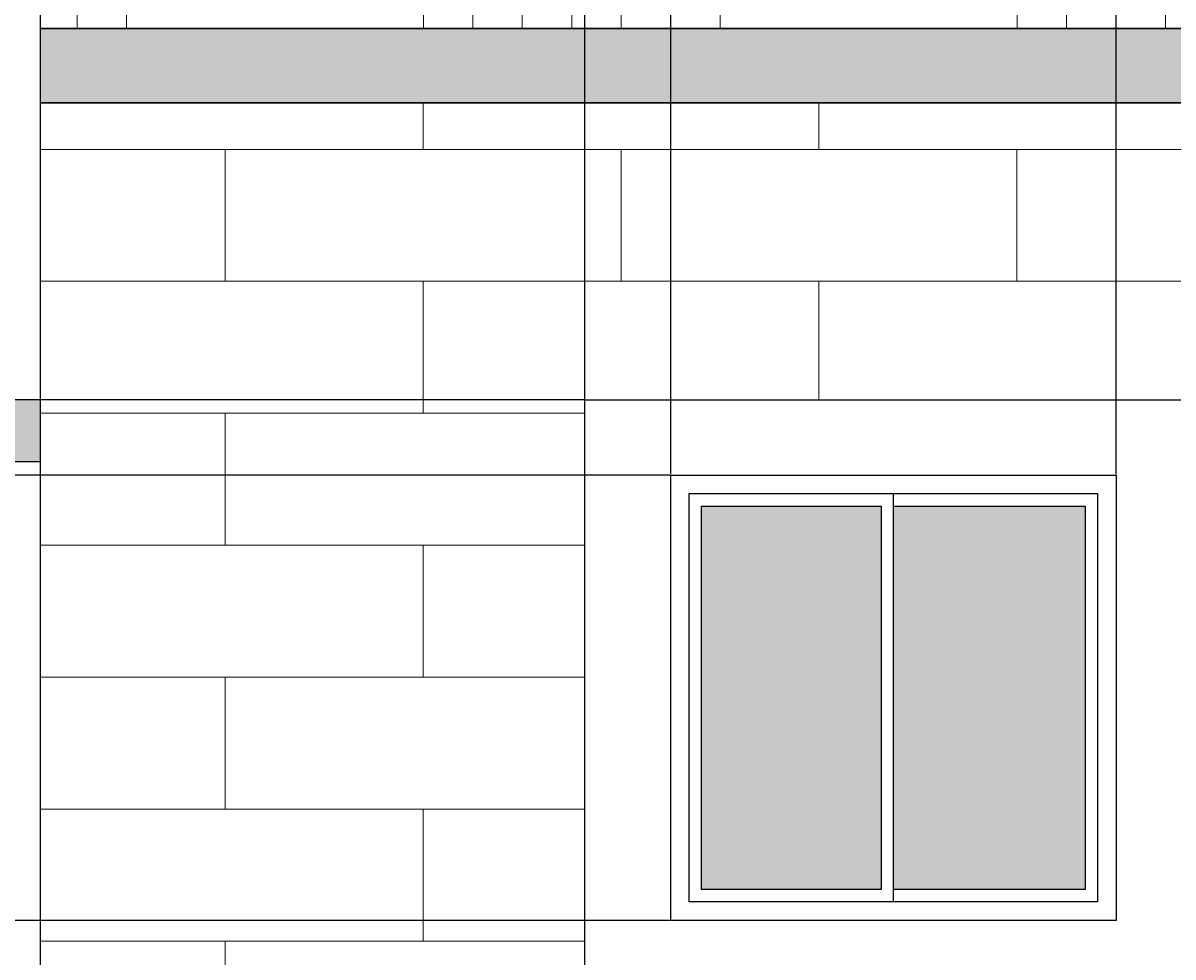
# Model space of a CAD drawing. Units: inches. Extents: x 37 to 824, y -700 to 234.
# Tile 4 of 77: x 160 to 253, y -535 to -459. Entities that reach past the tile are written whole.
import ezdxf

# ---------------------------------------------------------------- set-up
doc = ezdxf.new("R2010")
doc.units = ezdxf.units.IN
doc.header["$MEASUREMENT"] = 0
for name, color, linetype, lineweight in [('A-ANNO-DIMS', 2, 'Continuous', 18), ('A-ELEV', 3, 'Continuous', 25), ('A-ELEV-PATT', 8, 'Continuous', 13), ('A-GLAZ', 4, 'Continuous', 25)]:
    doc.layers.add(name, color=color, linetype=linetype, lineweight=lineweight)
doc.styles.get("Standard").update_dxf_attribs({"font": 'arial.ttf'})
doc.dimstyles.get("Standard").update_dxf_attribs({"dimtxt": 0.18, "dimasz": 0.18, "dimexe": 0.18, "dimexo": 0.0625, "dimgap": 0.09, "dimtad": 0, "dimtih": 1, "dimtoh": 1, "dimdec": 1, "dimzin": 0, "dimdsep": 46, "dimlunit": 4, "dimtxsty": 'Standard', "dimcen": 0.09, "dimadec": 0, "dimazin": 0, "dimtfac": 1, "dimtdec": 1, "dimtofl": 0, "dimtmove": 0, "dimatfit": 3, "dimfxl": 1, "dimtolj": 1, "dimtzin": 0, "dimarcsym": 0})

# ---------------------------------------------------------------- blocks, each defined once
blk = doc.blocks.new('*U11')
for p, q in [((1.5, 1.5), (1.5, 34.5)), ((1.5, 34.5), (18, 34.5)), ((18, 1.5), (18, 34.5)), ((18, 34.5), (34.5, 34.5)), ((34.5, 34.5), (34.5, 1.5)), ((18, 1.5), (1.5, 1.5)), ((34.5, 1.5), (18, 1.5))]:
    blk.add_line(p, q)
blk.add_lwpolyline([(0, 0), (0, 36), (36, 36), (36, 0)], close=True)
for points in [[(17, 33.5), (17, 2.5), (2.5, 2.5), (2.5, 33.5), (17, 33.5)], [(18, 33.5), (33.5, 33.5), (33.5, 2.5), (18, 2.5)]]:
    blk.add_lwpolyline(points)
blk = doc.blocks.new('*D94')
at = {"layer": 'A-ANNO-DIMS', "color": 0, "lineweight": -2, "ltscale": 0.5, "transparency": 16777216}
for p, q in [((205.077, -489.565), (205.077, -378.38)), ((212.025, -495.652), (212.025, -378.38)), ((205.257, -378.56), (208.222, -378.56)), ((211.845, -378.56), (208.88, -378.56))]:
    blk.add_line(p, q, dxfattribs=at)
at = {"layer": 'A-ANNO-DIMS', "color": 0, "ltscale": 0.5, "transparency": 16777216}
for points in [[(205.257, -378.53), (205.257, -378.59), (205.077, -378.56)], [(211.845, -378.53), (211.845, -378.59), (212.025, -378.56)]]:
    blk.add_solid(points, dxfattribs=at)
at = {"layer": 'Defpoints', "color": 0, "ltscale": 0.5, "transparency": 16777216}
for p in [(212.025, -378.56), (205.077, -489.627), (212.025, -495.714)]:
    blk.add_point(p, dxfattribs=at)
at = {"layer": 'A-ANNO-DIMS', "color": 0, "ltscale": 0.5, "transparency": 16777216, "insert": (208.551, -378.56), "char_height": 0.18, "attachment_point": 5}
blk.add_mtext('\\A1;0\'-7"', dxfattribs=at)
blk = doc.blocks.new('*D95')
at = {"layer": 'A-ANNO-DIMS', "color": 0, "lineweight": -2, "ltscale": 0.5, "transparency": 16777216}
for p, q in [((212.025, -495.652), (212.025, -378.38)), ((248.025, -495.652), (248.025, -378.38)), ((212.205, -378.56), (229.696, -378.56)), ((247.845, -378.56), (230.354, -378.56))]:
    blk.add_line(p, q, dxfattribs=at)
at = {"layer": 'A-ANNO-DIMS', "color": 0, "ltscale": 0.5, "transparency": 16777216}
for points in [[(212.205, -378.53), (212.205, -378.59), (212.025, -378.56)], [(247.845, -378.53), (247.845, -378.59), (248.025, -378.56)]]:
    blk.add_solid(points, dxfattribs=at)
at = {"layer": 'Defpoints', "color": 0, "ltscale": 0.5, "transparency": 16777216}
for p in [(248.025, -378.56), (212.025, -495.714), (248.025, -495.714)]:
    blk.add_point(p, dxfattribs=at)
at = {"layer": 'A-ANNO-DIMS', "color": 0, "ltscale": 0.5, "transparency": 16777216, "insert": (230.025, -378.56), "char_height": 0.18, "attachment_point": 5}
blk.add_mtext('\\A1;3\'-0"', dxfattribs=at)
blk = doc.blocks.new('*D96')
at = {"layer": 'A-ANNO-DIMS', "color": 0, "lineweight": -2, "ltscale": 0.5, "transparency": 16777216}
for p, q in [((205.015, -489.627), (36.851, -489.627)), ((37.031, -489.807), (37.031, -492.489)), ((37.031, -495.534), (37.031, -492.853)), ((211.963, -495.714), (36.851, -495.714))]:
    blk.add_line(p, q, dxfattribs=at)
at = {"layer": 'A-ANNO-DIMS', "color": 0, "ltscale": 0.5, "transparency": 16777216}
for points in [[(37.001, -489.807), (37.061, -489.807), (37.031, -489.627)], [(37.001, -495.534), (37.061, -495.534), (37.031, -495.714)]]:
    blk.add_solid(points, dxfattribs=at)
at = {"layer": 'Defpoints', "color": 0, "ltscale": 0.5, "transparency": 16777216}
for p in [(205.077, -489.627), (37.031, -495.714), (212.025, -495.714)]:
    blk.add_point(p, dxfattribs=at)
at = {"layer": 'A-ANNO-DIMS', "color": 0, "ltscale": 0.5, "transparency": 16777216, "insert": (37.031, -492.671), "char_height": 0.18, "attachment_point": 5}
blk.add_mtext('\\A1;0\'-6"', dxfattribs=at)
blk = doc.blocks.new('*D97')
at = {"layer": 'A-ANNO-DIMS', "color": 0, "lineweight": -2, "ltscale": 0.5, "transparency": 16777216}
for p, q in [((211.963, -495.714), (36.851, -495.714)), ((37.031, -495.894), (37.031, -513.532)), ((37.031, -531.534), (37.031, -513.896)), ((211.963, -531.714), (36.851, -531.714))]:
    blk.add_line(p, q, dxfattribs=at)
at = {"layer": 'A-ANNO-DIMS', "color": 0, "ltscale": 0.5, "transparency": 16777216}
for points in [[(37.001, -495.894), (37.061, -495.894), (37.031, -495.714)], [(37.001, -531.534), (37.061, -531.534), (37.031, -531.714)]]:
    blk.add_solid(points, dxfattribs=at)
at = {"layer": 'Defpoints', "color": 0, "ltscale": 0.5, "transparency": 16777216}
for p in [(212.025, -495.714), (37.031, -531.714), (212.025, -531.714)]:
    blk.add_point(p, dxfattribs=at)
at = {"layer": 'A-ANNO-DIMS', "color": 0, "ltscale": 0.5, "transparency": 16777216, "insert": (37.031, -513.714), "char_height": 0.18, "attachment_point": 5}
blk.add_mtext('\\A1;3\'-0"', dxfattribs=at)

msp = doc.modelspace()

# ---------------------------------------------------------------- hatches: boundary and pattern name
at = {"layer": 'A-ELEV-PATT', "ltscale": 0.5}
h = msp.add_hatch(dxfattribs=at)
h.set_pattern_fill('AR-PARQ1', color=256, scale=2)
h.paths.add_polyline_path([(428.077, -423.627), (161.077, -423.627), (161.077, -459.627), (428.077, -459.627)])
h = msp.add_hatch(color=256, dxfattribs=at)
h.dxf.hatch_style = 1
h.paths.add_polyline_path([(161.077, -459.627), (161.077, -465.627), (428.077, -465.627), (428.077, -459.627)])
h.paths.add_polyline_path([(229.025, -498.214), (214.525, -498.214), (214.525, -529.214), (229.025, -529.214)])
h.paths.add_polyline_path([(245.525, -498.214), (230.025, -498.214), (230.025, -529.214), (245.525, -529.214)])
h.paths.add_polyline_path([(315.196, -574.007), (341.196, -574.007), (341.196, -505.03), (315.196, -505.03)])
h = msp.add_hatch(dxfattribs=at)
h.set_pattern_fill('AR-BRSTD', color=256, scale=4)
h.paths.add_polyline_path([(299.077, -489.627), (358.132, -489.627), (358.132, -585.627), (428.077, -585.627), (428.077, -465.627), (161.077, -465.627), (161.077, -585.627), (299.077, -585.627)])
h.paths.add_polyline_path([(205.077, -537.627), (205.077, -489.627), (255.077, -489.627), (255.077, -537.627)], flags=16)
h = msp.add_hatch(color=256, dxfattribs=at)
h.dxf.hatch_style = 1
h.paths.add_polyline_path([(440.077, -489.627), (428.077, -489.627), (428.077, -494.627), (440.077, -494.627)])
h.paths.add_polyline_path([(161.077, -489.627), (149.077, -489.627), (149.077, -494.627), (161.077, -494.627)])

# ---------------------------------------------------------------- linework, layer by layer
at = {"layer": 'A-ELEV', "ltscale": 0.5}
for p, q in [((161.077, -489.627), (149.077, -489.627)), ((149.077, -494.627), (161.077, -494.627))]:
    msp.add_line(p, q, dxfattribs=at)
for points in [[(161.077, -423.627), (428.077, -423.627), (428.077, -459.627), (161.077, -459.627)], [(161.077, -459.627), (428.077, -459.627), (428.077, -465.627), (161.077, -465.627)], [(161.077, -465.627), (428.077, -465.627), (428.077, -585.627), (161.077, -585.627)], [(205.077, -489.627), (255.077, -489.627), (255.077, -537.627), (205.077, -537.627)]]:
    msp.add_lwpolyline(points, close=True, dxfattribs=at)

# ---------------------------------------------------------------- block references
at = {"layer": 'A-GLAZ'}
msp.add_blockref('*U11', (212.025, -531.714), dxfattribs=at)

# ---------------------------------------------------------------- dimensions: what is measured, and where the dimension line sits
at = {"layer": 'A-ANNO-DIMS', "ltscale": 0.5}
for base, p1, p2, picture, middle in [((212.025, -378.56), (205.077, -489.627), (212.025, -495.714), '*D94', (208.551, -378.56)), ((248.025, -378.56), (212.025, -495.714), (248.025, -495.714), '*D95', (230.025, -378.56))]:
    dim = msp.add_linear_dim(base=base, p1=p1, p2=p2, dimstyle='Standard', override={"dimdec": 1, "dimlfac": 1, "dimrnd": 0, "dimzin": 1, "dimdsep": 46, "dimlunit": 4, "dimfrac": 2}, dxfattribs=at)
    dim.commit()
    dim.dimension.update_dxf_attribs({"geometry": picture, "text_midpoint": middle})
for base, p1, p2, picture, middle in [((37.031, -495.714), (205.077, -489.627), (212.025, -495.714), '*D96', (37.031, -492.671)), ((37.031, -531.714), (212.025, -495.714), (212.025, -531.714), '*D97', (37.031, -513.714))]:
    dim = msp.add_linear_dim(base=base, p1=p1, p2=p2, angle=90, dimstyle='Standard', override={"dimdec": 1, "dimlfac": 1, "dimrnd": 0, "dimzin": 1, "dimdsep": 46, "dimlunit": 4, "dimfrac": 2}, dxfattribs=at)
    dim.commit()
    dim.dimension.update_dxf_attribs({"geometry": picture, "text_midpoint": middle})

doc.saveas('drawing.dxf')
